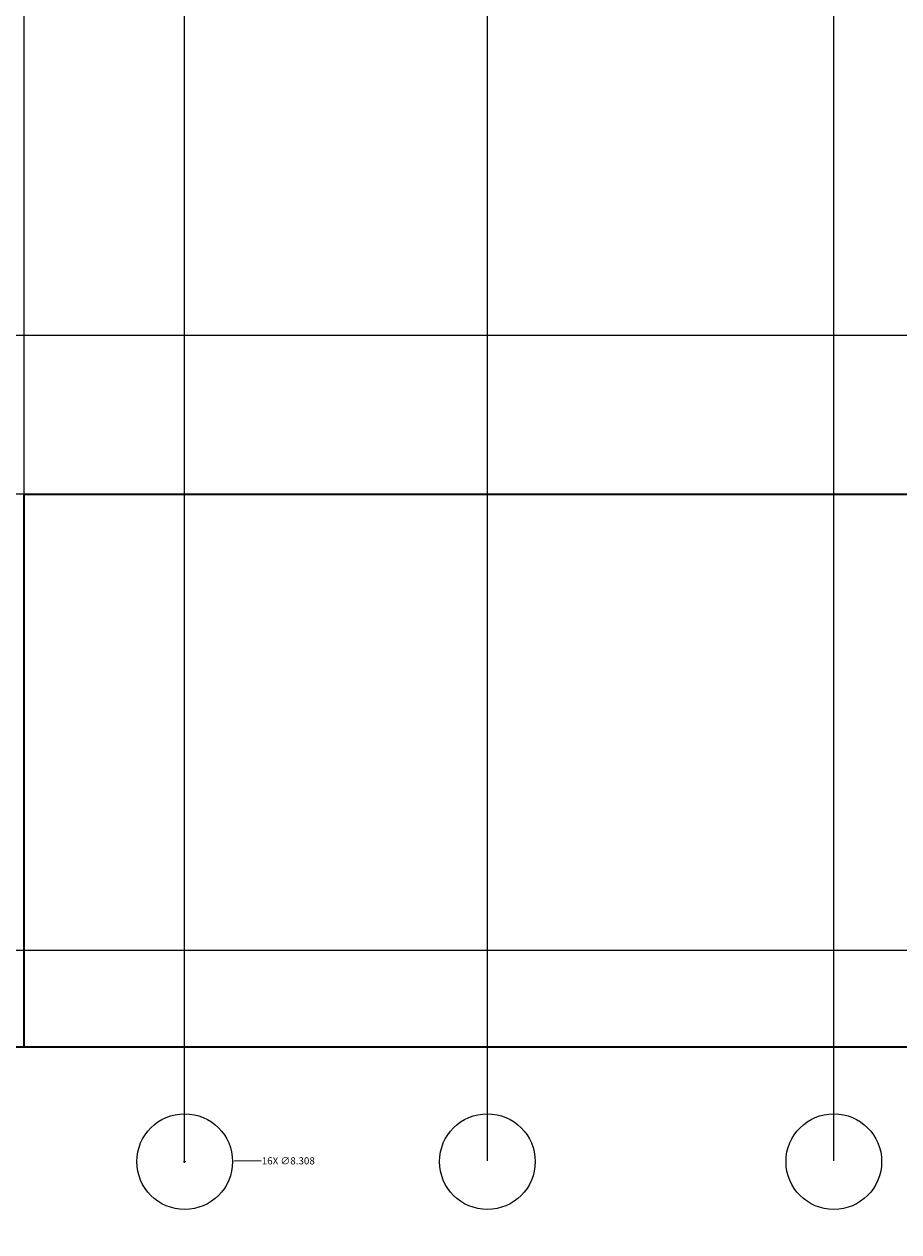
# Model space of a CAD drawing. Units: inches. Extents: x -13 to 809, y 112 to 656.
# Tile 29 of 55: x 107 to 183, y 446 to 551. Entities that reach past the tile are written whole.
import ezdxf

# ---------------------------------------------------------------- set-up
doc = ezdxf.new("R2010")
doc.units = ezdxf.units.IN
doc.header["$MEASUREMENT"] = 0
for name, color, linetype, lineweight in [('A-ANNO-DIMS', 2, 'Continuous', 18), ('A-ELEV', 7, 'Continuous', 35), ('A-ELEV-OTLN', 7, 'Continuous', 18)]:
    doc.layers.add(name, color=color, linetype=linetype, lineweight=lineweight)
doc.styles.get("Standard").update_dxf_attribs({"font": 'arial.ttf'})
doc.dimstyles.get("Standard").update_dxf_attribs({"dimtxt": 0.625, "dimasz": 0.18, "dimexe": 0.18, "dimexo": 0.0625, "dimgap": 0.09, "dimtad": 0, "dimtih": 1, "dimtoh": 1, "dimdec": 4, "dimzin": 0, "dimdsep": 46, "dimlunit": 4, "dimtxsty": 'Standard', "dimcen": 0.09, "dimadec": 0, "dimazin": 0, "dimtfac": 1, "dimtdec": 4, "dimtofl": 0, "dimtmove": 0, "dimatfit": 3, "dimfxl": 1, "dimtolj": 1, "dimtzin": 0, "dimarcsym": 0})

# ---------------------------------------------------------------- blocks, each defined once
blk = doc.blocks.new('*D23')
at = {"layer": 'A-ANNO-DIMS', "color": 0, "lineweight": -2, "transparency": 16777216}
for p, q in [((107.26, 510.58), (107.26, 655.96)), ((107.44, 655.78), (198.73, 655.78)), ((292.74, 655.78), (201.45, 655.78)), ((292.92, 569.3), (292.92, 655.96))]:
    blk.add_line(p, q, dxfattribs=at)
at = {"layer": 'A-ANNO-DIMS', "color": 0, "transparency": 16777216}
for points in [[(107.44, 655.81), (107.44, 655.75), (107.26, 655.78)], [(292.74, 655.81), (292.74, 655.75), (292.92, 655.78)]]:
    blk.add_solid(points, dxfattribs=at)
at = {"layer": 'Defpoints', "color": 0, "transparency": 16777216}
for p in [(292.92, 655.78), (292.92, 569.24), (107.26, 510.52)]:
    blk.add_point(p, dxfattribs=at)
at = {"layer": 'A-ANNO-DIMS', "color": 0, "transparency": 16777216, "insert": (200.09, 655.78), "char_height": 0.625, "attachment_point": 5}
blk.add_mtext('\\A1;185.66', dxfattribs=at)
blk = doc.blocks.new('*D36')
at = {"layer": 'A-ANNO-DIMS', "color": 0, "lineweight": -2, "transparency": 16777216}
for p, q in [((311.64, 569.24), (-12.1, 569.24)), ((-11.92, 569.06), (-11.92, 540.29)), ((-11.92, 510.7), (-11.92, 539.47)), ((107.2, 510.52), (-12.1, 510.52))]:
    blk.add_line(p, q, dxfattribs=at)
at = {"layer": 'A-ANNO-DIMS', "color": 0, "transparency": 16777216}
for points in [[(-11.95, 569.06), (-11.89, 569.06), (-11.92, 569.24)], [(-11.95, 510.7), (-11.89, 510.7), (-11.92, 510.52)]]:
    blk.add_solid(points, dxfattribs=at)
at = {"layer": 'Defpoints', "color": 0, "transparency": 16777216}
for p in [(-11.92, 569.24), (311.7, 569.24), (107.26, 510.52)]:
    blk.add_point(p, dxfattribs=at)
at = {"layer": 'A-ANNO-DIMS', "color": 0, "transparency": 16777216, "insert": (-11.92, 539.88), "char_height": 0.625, "attachment_point": 5}
blk.add_mtext('\\A1;58.72', dxfattribs=at)
blk = doc.blocks.new('*D39')
at = {"layer": 'A-ANNO-DIMS', "color": 0, "lineweight": -2, "transparency": 16777216}
for p, q in [((341.34, 524.28), (-12.1, 524.28)), ((-11.92, 524.1), (-11.92, 406.78)), ((-11.92, 288.63), (-11.92, 405.96)), ((341.34, 288.45), (-12.1, 288.45))]:
    blk.add_line(p, q, dxfattribs=at)
at = {"layer": 'A-ANNO-DIMS', "color": 0, "transparency": 16777216}
for points in [[(-11.95, 524.1), (-11.89, 524.1), (-11.92, 524.28)], [(-11.95, 288.63), (-11.89, 288.63), (-11.92, 288.45)]]:
    blk.add_solid(points, dxfattribs=at)
at = {"layer": 'Defpoints', "color": 0, "transparency": 16777216}
for p in [(-11.92, 524.28), (341.41, 524.28), (341.41, 288.45)]:
    blk.add_point(p, dxfattribs=at)
at = {"layer": 'A-ANNO-DIMS', "color": 0, "transparency": 16777216, "insert": (-11.92, 406.37), "char_height": 0.625, "attachment_point": 5}
blk.add_mtext('\\A1;235.83', dxfattribs=at)
blk = doc.blocks.new('*D43')
at = {"layer": 'A-ANNO-DIMS', "color": 0, "lineweight": -2, "transparency": 16777216}
for p, q in [((471.04, 470.88), (-12.1, 470.88)), ((-11.92, 470.7), (-11.92, 443.28)), ((-11.92, 415.04), (-11.92, 442.46)), ((471.04, 414.86), (-12.1, 414.86))]:
    blk.add_line(p, q, dxfattribs=at)
at = {"layer": 'A-ANNO-DIMS', "color": 0, "transparency": 16777216}
for points in [[(-11.95, 470.7), (-11.89, 470.7), (-11.92, 470.88)], [(-11.95, 415.04), (-11.89, 415.04), (-11.92, 414.86)]]:
    blk.add_solid(points, dxfattribs=at)
at = {"layer": 'Defpoints', "color": 0, "transparency": 16777216}
for p in [(-11.92, 470.88), (471.1, 470.88), (471.1, 414.86)]:
    blk.add_point(p, dxfattribs=at)
at = {"layer": 'A-ANNO-DIMS', "color": 0, "transparency": 16777216, "insert": (-11.92, 442.87), "char_height": 0.625, "attachment_point": 5}
blk.add_mtext('\\A1;56.02', dxfattribs=at)
blk = doc.blocks.new('*D93')
at = {"layer": 'A-ANNO-DIMS', "color": 0, "lineweight": -2, "transparency": 16777216}
for p, q in [((121.11, 452.56), (121.29, 452.56)), ((121.2, 452.47), (121.2, 452.65)), ((127.85, 452.63), (125.54, 452.61))]:
    blk.add_line(p, q, dxfattribs=at)
at = {"layer": 'A-ANNO-DIMS', "color": 0, "transparency": 16777216}
blk.add_solid([(125.54, 452.64), (125.54, 452.58), (125.36, 452.6)], dxfattribs=at)
at = {"layer": 'Defpoints', "color": 0, "transparency": 16777216}
for p in [(117.05, 452.52), (125.36, 452.6)]:
    blk.add_point(p, dxfattribs=at)
at = {"layer": 'A-ANNO-DIMS', "color": 0, "transparency": 16777216, "insert": (130.2, 452.63), "char_height": 0.625, "attachment_point": 5}
blk.add_mtext('\\A1;16X ∅8.308', dxfattribs=at)
blk = doc.blocks.new('*D95')
at = {"layer": 'A-ANNO-DIMS', "color": 0, "lineweight": -2, "transparency": 16777216}
for p, q in [((95.05, 462.58), (95.05, 655.96)), ((95.23, 655.78), (106.98, 655.78)), ((121.02, 655.78), (109.28, 655.78)), ((121.2, 452.63), (121.2, 655.96))]:
    blk.add_line(p, q, dxfattribs=at)
at = {"layer": 'A-ANNO-DIMS', "color": 0, "transparency": 16777216}
for points in [[(95.23, 655.81), (95.23, 655.75), (95.05, 655.78)], [(121.02, 655.81), (121.02, 655.75), (121.2, 655.78)]]:
    blk.add_solid(points, dxfattribs=at)
at = {"layer": 'Defpoints', "color": 0, "transparency": 16777216}
for p in [(121.2, 655.78), (95.05, 462.52), (121.2, 452.56)]:
    blk.add_point(p, dxfattribs=at)
at = {"layer": 'A-ANNO-DIMS', "color": 0, "transparency": 16777216, "insert": (108.13, 655.78), "char_height": 0.625, "attachment_point": 5}
blk.add_mtext('\\A1;26.16', dxfattribs=at)
blk = doc.blocks.new('*D96')
at = {"layer": 'A-ANNO-DIMS', "color": 0, "lineweight": -2, "transparency": 16777216}
for p, q in [((121.2, 452.63), (121.2, 655.96)), ((121.38, 655.78), (133.2, 655.78)), ((147.31, 655.78), (135.5, 655.78)), ((147.49, 452.63), (147.49, 655.96))]:
    blk.add_line(p, q, dxfattribs=at)
at = {"layer": 'A-ANNO-DIMS', "color": 0, "transparency": 16777216}
for points in [[(121.38, 655.81), (121.38, 655.75), (121.2, 655.78)], [(147.31, 655.81), (147.31, 655.75), (147.49, 655.78)]]:
    blk.add_solid(points, dxfattribs=at)
at = {"layer": 'Defpoints', "color": 0, "transparency": 16777216}
for p in [(147.49, 655.78), (121.2, 452.56), (147.49, 452.56)]:
    blk.add_point(p, dxfattribs=at)
at = {"layer": 'A-ANNO-DIMS', "color": 0, "transparency": 16777216, "insert": (134.35, 655.78), "char_height": 0.625, "attachment_point": 5}
blk.add_mtext('\\A1;26.29', dxfattribs=at)
blk = doc.blocks.new('*D97')
at = {"layer": 'A-ANNO-DIMS', "color": 0, "lineweight": -2, "transparency": 16777216}
for p, q in [((147.49, 452.63), (147.49, 655.96)), ((147.67, 655.78), (161.39, 655.78)), ((177.41, 655.78), (163.68, 655.78)), ((177.59, 452.63), (177.59, 655.96))]:
    blk.add_line(p, q, dxfattribs=at)
at = {"layer": 'A-ANNO-DIMS', "color": 0, "transparency": 16777216}
for points in [[(147.67, 655.81), (147.67, 655.75), (147.49, 655.78)], [(177.41, 655.81), (177.41, 655.75), (177.59, 655.78)]]:
    blk.add_solid(points, dxfattribs=at)
at = {"layer": 'Defpoints', "color": 0, "transparency": 16777216}
for p in [(177.59, 655.78), (147.49, 452.56), (177.59, 452.56)]:
    blk.add_point(p, dxfattribs=at)
at = {"layer": 'A-ANNO-DIMS', "color": 0, "transparency": 16777216, "insert": (162.54, 655.78), "char_height": 0.625, "attachment_point": 5}
blk.add_mtext('\\A1;30.09', dxfattribs=at)
blk = doc.blocks.new('*D98')
at = {"layer": 'A-ANNO-DIMS', "color": 0, "lineweight": -2, "transparency": 16777216}
for p, q in [((177.59, 452.63), (177.59, 655.96)), ((177.77, 655.78), (189.7, 655.78)), ((204.42, 655.78), (192.49, 655.78)), ((204.6, 452.63), (204.6, 655.96))]:
    blk.add_line(p, q, dxfattribs=at)
at = {"layer": 'A-ANNO-DIMS', "color": 0, "transparency": 16777216}
for points in [[(177.77, 655.81), (177.77, 655.75), (177.59, 655.78)], [(204.42, 655.81), (204.42, 655.75), (204.6, 655.78)]]:
    blk.add_solid(points, dxfattribs=at)
at = {"layer": 'Defpoints', "color": 0, "transparency": 16777216}
for p in [(204.6, 655.78), (177.59, 452.56), (204.6, 452.56)]:
    blk.add_point(p, dxfattribs=at)
at = {"layer": 'A-ANNO-DIMS', "color": 0, "transparency": 16777216, "insert": (191.09, 655.78), "char_height": 0.625, "attachment_point": 5}
blk.add_mtext('\\A1;27.017', dxfattribs=at)

msp = doc.modelspace()

# ---------------------------------------------------------------- linework, layer by layer
at = {"layer": 'A-ELEV'}
for p, q in [((107.2588, 498.5199), (107.2588, 510.5199)), ((107.2588, 510.5199), (341.4072, 510.5199)), ((107.2588, 462.5199), (107.2588, 498.5199)), ((95.0469, 462.5199), (337.5074, 462.5199))]:
    msp.add_line(p, q, dxfattribs=at)
at = {"layer": 'A-ELEV-OTLN'}
for centre in [(121.2048, 452.5629), (147.4935, 452.5629), (177.5857, 452.5629)]:
    msp.add_circle(centre, 4.1542, dxfattribs=at)

# ---------------------------------------------------------------- dimensions: what is measured, and where the dimension line sits
at = {"layer": 'A-ANNO-DIMS'}
for base, p1, p2, override, picture, middle in [((121.2048, 655.7828), (95.0469, 462.5199), (121.2048, 452.5629), {"dimdec": 2, "dimlfac": 1, "dimrnd": 0, "dimzin": 0, "dimdsep": 46, "dimlunit": 2}, '*D95', (108.1258, 655.7828)), ((292.923, 655.7828), (107.2588, 510.5199), (292.923, 569.2414), {"dimdec": 2, "dimlfac": 1, "dimrnd": 0, "dimzin": 0, "dimdsep": 46, "dimlunit": 2}, '*D23', (200.0909, 655.7828)), ((147.4935, 655.7828), (121.2048, 452.5629), (147.4935, 452.5629), {"dimdec": 2, "dimlfac": 1, "dimrnd": 0, "dimzin": 0, "dimdsep": 46, "dimlunit": 2}, '*D96', (134.3491, 655.7828)), ((177.5857, 655.7828), (147.4935, 452.5629), (177.5857, 452.5629), {"dimdec": 2, "dimlfac": 1, "dimrnd": 0, "dimzin": 0, "dimdsep": 46, "dimlunit": 2}, '*D97', (162.5396, 655.7828)), ((204.6029, 655.7828), (177.5857, 452.5629), (204.6029, 452.5629), {"dimdec": 3, "dimlfac": 1, "dimrnd": 0, "dimzin": 0, "dimdsep": 46, "dimlunit": 2}, '*D98', (191.0943, 655.7828))]:
    dim = msp.add_linear_dim(base=base, p1=p1, p2=p2, dimstyle='Standard', override=override, dxfattribs=at)
    dim.commit()
    dim.dimension.update_dxf_attribs({"geometry": picture, "text_midpoint": middle})
for base, p1, p2, picture, middle in [((-11.9191, 569.2414), (107.2588, 510.5199), (311.6991, 569.2414), '*D36', (-11.9191, 539.8806)), ((-11.9191, 524.281), (341.4072, 288.4508), (341.4072, 524.281), '*D39', (-11.9191, 406.3659)), ((-11.9191, 470.8765), (471.0998, 414.8594), (471.0998, 470.8765), '*D43', (-11.9191, 442.8679))]:
    dim = msp.add_linear_dim(base=base, p1=p1, p2=p2, angle=90, dimstyle='Standard', override={"dimdec": 2, "dimlfac": 1, "dimrnd": 0, "dimzin": 0, "dimdsep": 46, "dimlunit": 2}, dxfattribs=at)
    dim.commit()
    dim.dimension.update_dxf_attribs({"geometry": picture, "text_midpoint": middle})
dim = msp.add_diameter_dim_2p(p1=(117.0507, 452.5223), p2=(125.3588, 452.6035), text='16X <>', dimstyle='Standard', override={"dimdec": 3, "dimlfac": 1, "dimrnd": 0, "dimzin": 0, "dimdsep": 46, "dimlunit": 2}, dxfattribs=at)
dim.commit()
dim.dimension.update_dxf_attribs({"geometry": '*D93', "text_midpoint": (127.8512, 452.6279), "dimtype": 163})

doc.saveas('drawing.dxf')
